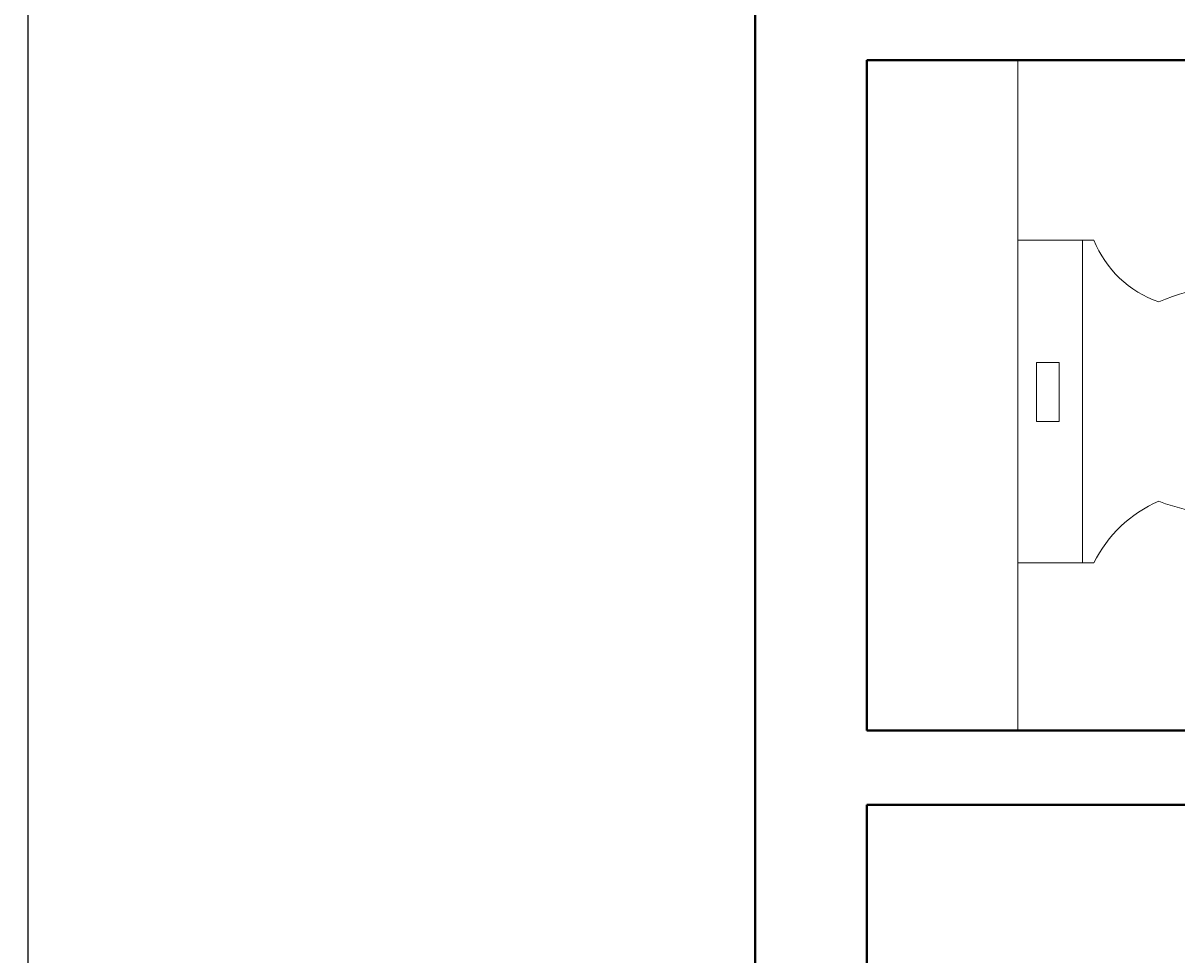
# Model space of a CAD drawing. Units: inches. Extents: x -46 to 1145, y -527 to 760.
# Tile 24 of 57: x -46 to 47, y 367 to 443. Entities that reach past the tile are written whole.
import ezdxf

# ---------------------------------------------------------------- set-up
doc = ezdxf.new("R2010")
doc.units = ezdxf.units.IN
doc.header["$MEASUREMENT"] = 0
for name, color, linetype, lineweight in [('A-ANNO-DIMS', 2, 'Continuous', 18), ('A-FLOR-CASE', 32, 'Continuous', 18), ('A-FLOR-FIXT', 9, 'Continuous', 18), ('WALLS', 4, 'Continuous', 40)]:
    doc.layers.add(name, color=color, linetype=linetype, lineweight=lineweight)
doc.styles.get("Standard").update_dxf_attribs({"font": 'arial.ttf'})
doc.dimstyles.get("Standard").update_dxf_attribs({"dimtxt": 0.18, "dimasz": 0.18, "dimexe": 0.18, "dimexo": 0.0625, "dimgap": 0.09, "dimtad": 0, "dimtih": 1, "dimtoh": 1, "dimdec": 0, "dimzin": 0, "dimdsep": 46, "dimlunit": 3, "dimtxsty": 'Standard', "dimcen": 0.09, "dimadec": 0, "dimazin": 0, "dimtfac": 1, "dimtdec": 0, "dimtofl": 0, "dimtmove": 0, "dimatfit": 3, "dimfxl": 1, "dimtolj": 1, "dimtzin": 0, "dimarcsym": 0})

# ---------------------------------------------------------------- blocks, each defined once
blk = doc.blocks.new('WATER-CLOSET')
for p, q in [((0, 0), (0, 26.013)), ((0, 26.013), (6.13, 26.013)), ((5.216, 21.037), (5.216, 26.013)), ((5.216, 26.013), (5.216, 0)), ((0, 0), (6.13, 0))]:
    blk.add_line(p, q)
blk.add_lwpolyline([(1.511, 11.402), (1.511, 16.163), (3.337, 16.163), (3.337, 11.402)], close=True)
blk.add_circle((19.793, 13.372), 1.752)
for centre, radius, start, end in [((14.154, 29.203), 8.635, 201.67821, 251.02588), ((18.35, 4.957), 17.539, 52.46164, 113.53592), ((22.519, 12.844), 8.873, 317.26823, 42.73177), ((18.329, 23.714), 19.999, 249.56451, 302.37094), ((15.403, -4.504), 10.309, 113.17039, 154.09473)]:
    blk.add_arc(centre, radius, start, end)
blk = doc.blocks.new('*D685')
at = {"layer": 'A-ANNO-DIMS', "color": 0, "lineweight": -2, "transparency": 16777216}
for p, q in [((183.501, 700.889), (-46.216, 700.889)), ((-46.036, 700.709), (-46.036, 116.385)), ((-46.036, -468.302), (-46.036, 116.021)), ((12.501, -468.482), (-46.216, -468.482))]:
    blk.add_line(p, q, dxfattribs=at)
at = {"layer": 'A-ANNO-DIMS', "color": 0, "transparency": 16777216}
for points in [[(-46.066, 700.709), (-46.006, 700.709), (-46.036, 700.889)], [(-46.066, -468.302), (-46.006, -468.302), (-46.036, -468.482)]]:
    blk.add_solid(points, dxfattribs=at)
at = {"layer": 'Defpoints', "color": 0, "transparency": 16777216}
for p in [(-46.036, 700.889), (183.564, 700.889), (12.564, -468.482)]:
    blk.add_point(p, dxfattribs=at)
at = {"layer": 'A-ANNO-DIMS', "color": 0, "transparency": 16777216, "insert": (-46.036, 116.203), "char_height": 0.18, "attachment_point": 5}
blk.add_mtext('\\A1;1169.4', dxfattribs=at)

msp = doc.modelspace()

# ---------------------------------------------------------------- linework, layer by layer
at = {"layer": 'A-FLOR-CASE'}
msp.add_line((33.7427, 439.5176), (33.7427, 385.5176), dxfattribs=at)
at = {"layer": 'WALLS'}
for p, q in [((12.5637, 659.5176), (12.5637, 221.5176)), ((21.5637, 385.5176), (21.5637, 439.5176)), ((131.5637, 439.5176), (21.5637, 439.5176)), ((131.5637, 385.5176), (21.5637, 385.5176)), ((183.5637, 379.5176), (21.5637, 379.5176)), ((21.5637, 379.5176), (21.5637, 230.5176))]:
    msp.add_line(p, q, dxfattribs=at)

# ---------------------------------------------------------------- block references
at = {"layer": 'A-FLOR-FIXT'}
msp.add_blockref('WATER-CLOSET', (33.743, 399.011), dxfattribs=at)

# ---------------------------------------------------------------- dimensions: what is measured, and where the dimension line sits
at = {"layer": 'A-ANNO-DIMS'}
dim = msp.add_linear_dim(base=(-46.0363, 700.8886), p1=(12.5637, -468.4824), p2=(183.5637, 700.8886), angle=90, dimstyle='Standard', override={"dimdec": 1, "dimlfac": 1, "dimrnd": 0, "dimzin": 0, "dimdsep": 46, "dimlunit": 2}, dxfattribs=at)
dim.commit()
dim.dimension.update_dxf_attribs({"geometry": '*D685', "text_midpoint": (-46.0363, 116.2031)})

doc.saveas('drawing.dxf')
